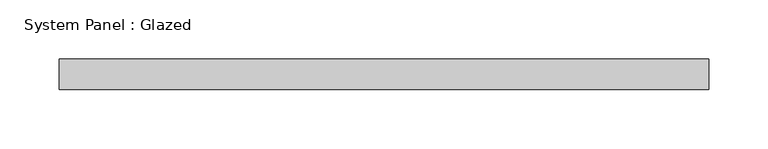
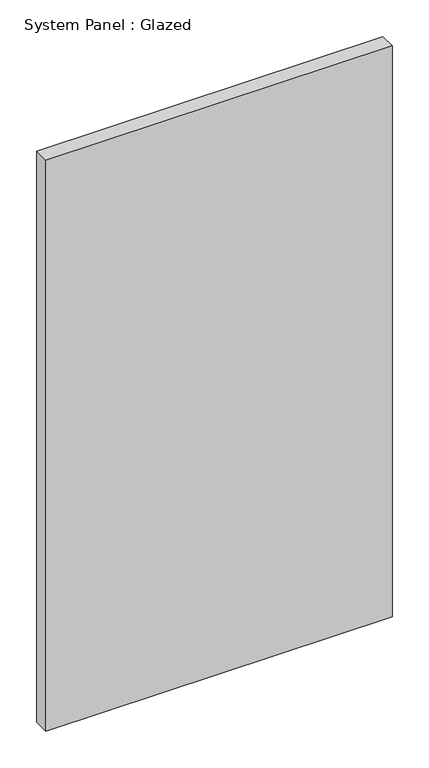
"""IFC4 building model written with IfcOpenShell, lengths in millimetres: plate geometry, System Panel : Glazed."""

from ifc_helpers import new_model, si_unit, origin, origin_with_axes, place, context, project, spatial, polyline, outline, extrude, source, transform, mapped, element, save


def system_panel_glazed_09326d9e(model_context):
    return source(origin(), model_context, "Body", "SweptSolid", [
        extrude(outline(polyline([(273.05, 19.05), (-273.05, 19.05), (-273.05, 44.45), (273.05, 44.45), (273.05, 19.05)])), origin_with_axes(), (0.0, 0.0, 1.0), 952.0990947),
    ])


if __name__ == "__main__":
    model = new_model("IFC4")
    model_context = context("Model", 3, world=origin())
    ifc_project = project(units=[si_unit("LENGTHUNIT", "METRE", prefix="MILLI")], contexts=[model_context])
    site = spatial("IfcSite", under=ifc_project)
    building = spatial("IfcBuilding", under=site)
    placement = place(None, origin())
    system_panel_glazed_shape = system_panel_glazed_09326d9e(model_context)
    element("IfcPlate", 1, ObjectType="System Panel : Glazed", at=placement, inside=building, context=model_context, shape_type="MappedRepresentation", body=[
        mapped(system_panel_glazed_shape, transform((0.0, 0.0, 0.0), x_axis=(1.0, 0.0, 0.0), y_axis=(0.0, 1.0, 0.0), z_axis=(0.0, 0.0, 1.0))),
    ])
    save(model, "model.ifc")

# Revit data of these elements
# Type "System Panel : Glazed"
#   Construction Type Id = "GSP4R"
#   Analytic Construction = "1/8 in Pilkington single glazing"
#   Visual Light Transmittance = 0.9
#   Solar Heat Gain Coefficient = 0.86
#   Heat Transfer Coefficient (U) = 1.18115 BTU/(h·ft²·°F)
#   Define Thermal Properties by = 1
# Element 1 (IfcPlate, "System Panel : Glazed")
#   Materials on its faces: "Glass"
# Materials
#   "Glass": class "Glass", colour RGB 0 128 192, transparency 0.75, Description = "Soda Lime Glass", Cost = 0
